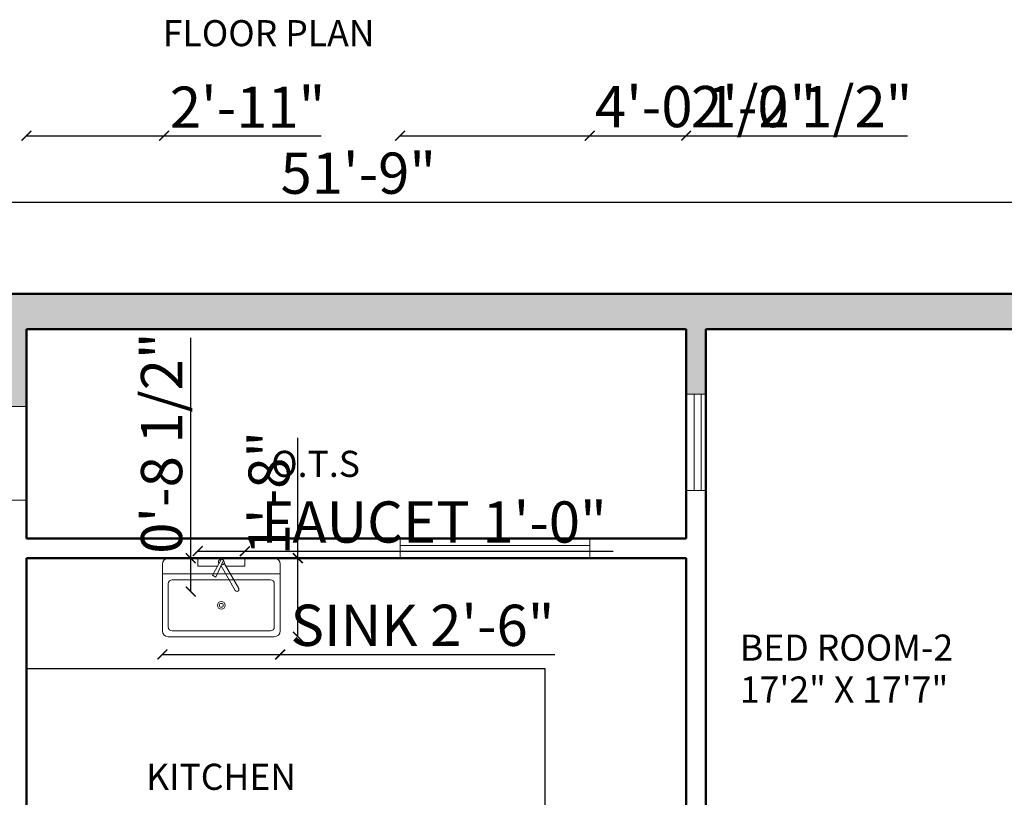
# Model space of a CAD drawing. Units: inches. Extents: x 1549 to 2410, y 1378 to 2139.
# Tile 5 of 6: x 1913 to 2164, y 1941 to 2139. Entities that reach past the tile are written whole.
import ezdxf

# ---------------------------------------------------------------- set-up
doc = ezdxf.new("R2010")
doc.units = ezdxf.units.IN
for name, color, linetype, lineweight in [('A-ANNO-DIMS', 2, 'Continuous', 18), ('A-ANNO-TEXT', 7, 'Continuous', 25), ('A-AREA-IDEN', 7, 'Continuous', 18), ('A-FLOR-CASE', 30, 'Continuous', 25), ('A-FLOR-FIXT', 9, 'Continuous', 18), ('A-WALL', 7, 'Continuous', 50), ('WINDOW', 2, 'Continuous', 18)]:
    doc.layers.add(name, color=color, linetype=linetype, lineweight=lineweight)
doc.layers.add('A-WALL-PATT', color=18, linetype='Continuous', lineweight=13, true_color=0x000000)
doc.styles.get("Standard").update_dxf_attribs({"font": 'arial.ttf'})
doc.dimstyles.new('ISO-25', dxfattribs={"dimtxt": 10.5, "dimasz": 2.5, "dimexe": 1.25, "dimexo": 0.625, "dimtad": 1, "dimdec": 0, "dimlunit": 4, "dimtxsty": 'Standard', "dimblk": 'ARCHTICK', "dimcen": 2.5, "dimse1": 1, "dimse2": 1, "dimclrd": 1, "dimclrt": 3, "dimadec": 0, "dimazin": 0, "dimtfac": 1, "dimtdec": 0, "dimtmove": 0, "dimatfit": 3, "dimfxl": 1, "dimarcsym": 0})

# ---------------------------------------------------------------- blocks, each defined once
blk = doc.blocks.new('Sink-single - 30 in top')
blk.add_line((-15, -3.999996), (15, -3.999996))
for points in [[(-13.5, 0), (13.5, 0)], [(-15, -18.499996), (-15, -1.5)], [(15, -1.5), (15, -18.499996)], [(-13.5, -17.499996), (-13.5, -6.499996)], [(-12.5, -5.499996), (12.5, -5.499996)], [(13.5, -6.499996), (13.5, -17.499996)], [(13.5, -19.999996), (-13.5, -19.999996)], [(12.5, -18.499996), (-12.5, -18.499996)]]:
    blk.add_lwpolyline(points)
for radius in [1, 0.5]:
    blk.add_circle((0, -11.999996), radius)
for centre, radius, start, end in [((-13.5, -1.5), 1.5, 90, 180), ((13.5, -1.5), 1.5, 0, 90), ((-12.5, -6.499996), 1, 90, 180), ((12.5, -6.499996), 1, 0, 90), ((-12.5, -17.499996), 1, 180, 270), ((12.5, -17.499996), 1, 270, 0), ((-13.5, -18.499996), 1.5, 180, 270), ((13.5, -18.499996), 1.5, 270, 0)]:
    blk.add_arc(centre, radius, start, end)
blk = doc.blocks.new('Faucet - single handle top')
for p, q in [((0.08, -0.26), (-2.26, -4.34)), ((-1.37, -4.79), (0.55, -0.5)), ((-0.06, -1.9), (3.57, -8.18)), ((4.43, -7.68), (0.72, -1.24)), ((-2.26, -4.34), (-1.37, -4.79))]:
    blk.add_line(p, q)
for points in [[(-0.92, -2), (-6, -2), (-6, 0), (6, 0), (6, -2), (1.16, -2)], [(-0.01, -2), (-0.12, -2)]]:
    blk.add_lwpolyline(points)
for centre, radius, start, end in [((0, -1), 0.75, 269.2246, 216.2304), ((4, -7.93), 0.5, 210, 30)]:
    blk.add_arc(centre, radius, start, end)
blk = doc.blocks.new('_ArchTick')
at = {"color": 0, "linetype": 'ByBlock', "const_width": 0.15}
blk.add_lwpolyline([(-0.5, -0.5), (0.5, 0.5)], dxfattribs=at)
blk = doc.blocks.new('*D13')
at = {"layer": 'A-ANNO-DIMS', "color": 0, "lineweight": -2, "transparency": 16777216}
blk.add_line((1688.62, 2092.38), (2309.62, 2092.38), dxfattribs=at)
at = {"layer": 'Defpoints', "color": 0, "transparency": 16777216}
for p in [(2309.62, 2092.38), (1688.62, 2069.01), (2309.62, 2069.01)]:
    blk.add_point(p, dxfattribs=at)
at = {"layer": 'A-ANNO-DIMS', "color": 0, "lineweight": -2, "transparency": 16777216, "xscale": 2.5, "yscale": 2.5, "zscale": 2.5, "rotation": 180}
blk.add_blockref('_ArchTick', (1688.62, 2092.38), dxfattribs=at)
at = {"layer": 'A-ANNO-DIMS', "color": 0, "lineweight": -2, "transparency": 16777216, "xscale": 2.5, "yscale": 2.5, "zscale": 2.5}
blk.add_blockref('_ArchTick', (2309.62, 2092.38), dxfattribs=at)
at = {"layer": 'A-ANNO-DIMS', "color": 0, "transparency": 16777216, "insert": (1999.12, 2098.36), "char_height": 10.5, "attachment_point": 5}
blk.add_mtext('51\'-9"', dxfattribs=at)
blk = doc.blocks.new('*D19')
at = {"layer": 'A-ANNO-DIMS', "color": 1, "lineweight": -2, "transparency": 16777216}
for p, q in [((1949.24, 1977.16), (1979.24, 1977.16)), ((1979.24, 1977.16), (2049.17, 1977.16))]:
    blk.add_line(p, q, dxfattribs=at)
at = {"layer": 'Defpoints', "color": 0, "transparency": 16777216}
for p in [(1949.24, 1981.66), (1979.24, 1981.66), (1979.24, 1977.16)]:
    blk.add_point(p, dxfattribs=at)
at = {"layer": 'A-ANNO-DIMS', "color": 1, "lineweight": -2, "transparency": 16777216, "xscale": 2.5, "yscale": 2.5, "zscale": 2.5, "rotation": 180}
blk.add_blockref('_ArchTick', (1949.24, 1977.16), dxfattribs=at)
at = {"layer": 'A-ANNO-DIMS', "color": 1, "lineweight": -2, "transparency": 16777216, "xscale": 2.5, "yscale": 2.5, "zscale": 2.5}
blk.add_blockref('_ArchTick', (1979.24, 1977.16), dxfattribs=at)
at = {"layer": 'A-ANNO-DIMS', "color": 3, "transparency": 16777216, "insert": (2015.46, 1983.22), "char_height": 10.5, "attachment_point": 5}
blk.add_mtext('SINK 2\'-6"', dxfattribs=at)
blk = doc.blocks.new('*D20')
at = {"layer": 'A-ANNO-DIMS', "color": 1, "lineweight": -2, "transparency": 16777216}
for p, q in [((1983.74, 2001.66), (1983.74, 2032.34)), ((1983.74, 1981.66), (1983.74, 2001.66))]:
    blk.add_line(p, q, dxfattribs=at)
at = {"layer": 'Defpoints', "color": 0, "transparency": 16777216}
for p in [(1979.24, 2001.66), (1983.74, 2001.66), (1979.24, 1981.66)]:
    blk.add_point(p, dxfattribs=at)
at = {"layer": 'A-ANNO-DIMS', "color": 1, "lineweight": -2, "transparency": 16777216, "xscale": 2.5, "yscale": 2.5, "zscale": 2.5}
for p, rotation in [((1983.74, 2001.66), 90), ((1983.74, 1981.66), 270)]:
    blk.add_blockref('_ArchTick', p, dxfattribs=dict(at, rotation=rotation))
at = {"layer": 'A-ANNO-DIMS', "color": 3, "transparency": 16777216, "insert": (1977.76, 2018.25), "char_height": 10.5, "attachment_point": 5, "rotation": 90}
blk.add_mtext('1\'-8"', dxfattribs=at)
blk = doc.blocks.new('*D21')
at = {"layer": 'A-ANNO-DIMS', "color": 1, "lineweight": -2, "transparency": 16777216}
for p, q in [((1958.24, 2003.46), (1970.24, 2003.46)), ((1970.24, 2003.46), (2064.06, 2003.46))]:
    blk.add_line(p, q, dxfattribs=at)
at = {"layer": 'Defpoints', "color": 0, "transparency": 16777216}
for p in [(1970.24, 2003.46), (1958.24, 2001.66), (1970.24, 2001.66)]:
    blk.add_point(p, dxfattribs=at)
at = {"layer": 'A-ANNO-DIMS', "color": 1, "lineweight": -2, "transparency": 16777216, "xscale": 2.5, "yscale": 2.5, "zscale": 2.5, "rotation": 180}
blk.add_blockref('_ArchTick', (1958.24, 2003.46), dxfattribs=at)
at = {"layer": 'A-ANNO-DIMS', "color": 1, "lineweight": -2, "transparency": 16777216, "xscale": 2.5, "yscale": 2.5, "zscale": 2.5}
blk.add_blockref('_ArchTick', (1970.24, 2003.46), dxfattribs=at)
at = {"layer": 'A-ANNO-DIMS', "color": 3, "transparency": 16777216, "insert": (2018.4, 2009.52), "char_height": 10.5, "attachment_point": 5}
blk.add_mtext('FAUCET 1\'-0"', dxfattribs=at)
blk = doc.blocks.new('*D22')
at = {"layer": 'A-ANNO-DIMS', "color": 1, "lineweight": -2, "transparency": 16777216}
for p, q in [((1956.44, 2001.66), (1956.44, 2057.79)), ((1956.44, 1993.17), (1956.44, 2001.66))]:
    blk.add_line(p, q, dxfattribs=at)
at = {"layer": 'Defpoints', "color": 0, "transparency": 16777216}
for p in [(1956.44, 2001.66), (1958.24, 2001.66), (1958.24, 1993.17)]:
    blk.add_point(p, dxfattribs=at)
at = {"layer": 'A-ANNO-DIMS', "color": 1, "lineweight": -2, "transparency": 16777216, "xscale": 2.5, "yscale": 2.5, "zscale": 2.5}
for p, rotation in [((1956.44, 2001.66), 90), ((1956.44, 1993.17), 270)]:
    blk.add_blockref('_ArchTick', p, dxfattribs=dict(at, rotation=rotation))
at = {"layer": 'A-ANNO-DIMS', "color": 3, "transparency": 16777216, "insert": (1950.39, 2030.98), "char_height": 10.5, "attachment_point": 5, "rotation": 90}
blk.add_mtext('0\'-8 1/2"', dxfattribs=at)
blk = doc.blocks.new('*D48')
at = {"layer": 'A-ANNO-DIMS', "color": 1, "lineweight": -2, "transparency": 16777216}
for p, q in [((2400.7, 2060.01), (2400.7, 2006.66)), ((2400.7, 2006.66), (2400.7, 1950.11))]:
    blk.add_line(p, q, dxfattribs=at)
at = {"layer": 'Defpoints', "color": 0, "transparency": 16777216}
for p in [(1914.62, 2060.01), (1914.62, 2006.66), (2400.7, 2006.66)]:
    blk.add_point(p, dxfattribs=at)
at = {"layer": 'A-ANNO-DIMS', "color": 1, "lineweight": -2, "transparency": 16777216, "xscale": 2.5, "yscale": 2.5, "zscale": 2.5}
for p, rotation in [((2400.7, 2060.01), 90), ((2400.7, 2006.66), 270)]:
    blk.add_blockref('_ArchTick', p, dxfattribs=dict(at, rotation=rotation))
at = {"layer": 'A-ANNO-DIMS', "color": 3, "transparency": 16777216, "insert": (2394.65, 1977.14), "char_height": 10.5, "attachment_point": 5, "rotation": 90}
blk.add_mtext('4\'-5 1/2"', dxfattribs=at)
blk = doc.blocks.new('*D51')
at = {"layer": 'A-ANNO-DIMS', "color": 1, "lineweight": -2, "transparency": 16777216}
for p, q in [((1648.37, 2001.66), (1648.37, 2033.51)), ((1648.37, 1973.56), (1648.37, 2001.66))]:
    blk.add_line(p, q, dxfattribs=at)
at = {"layer": 'Defpoints', "color": 0, "transparency": 16777216}
for p in [(1648.37, 2001.66), (1914.62, 2001.66), (1914.62, 1973.56)]:
    blk.add_point(p, dxfattribs=at)
at = {"layer": 'A-ANNO-DIMS', "color": 1, "lineweight": -2, "transparency": 16777216, "xscale": 2.5, "yscale": 2.5, "zscale": 2.5}
for p, rotation in [((1648.37, 2001.66), 90), ((1648.37, 1973.56), 270)]:
    blk.add_blockref('_ArchTick', p, dxfattribs=dict(at, rotation=rotation))
at = {"layer": 'A-ANNO-DIMS', "color": 3, "transparency": 16777216, "insert": (1642.47, 2018.83), "char_height": 10.5, "attachment_point": 5, "rotation": 90}
blk.add_mtext('2\'-4"', dxfattribs=at)
blk = doc.blocks.new('*D53')
at = {"layer": 'A-ANNO-DIMS', "color": 1, "lineweight": -2, "transparency": 16777216}
for p, q in [((2009.78, 2109.26), (2058.05, 2109.26)), ((2058.05, 2109.26), (2114.6, 2109.26))]:
    blk.add_line(p, q, dxfattribs=at)
at = {"layer": 'Defpoints', "color": 0, "transparency": 16777216}
for p in [(2058.05, 2109.26), (2009.78, 2006.66), (2058.05, 2006.66)]:
    blk.add_point(p, dxfattribs=at)
at = {"layer": 'A-ANNO-DIMS', "color": 1, "lineweight": -2, "transparency": 16777216, "xscale": 2.5, "yscale": 2.5, "zscale": 2.5, "rotation": 180}
blk.add_blockref('_ArchTick', (2009.78, 2109.26), dxfattribs=at)
at = {"layer": 'A-ANNO-DIMS', "color": 1, "lineweight": -2, "transparency": 16777216, "xscale": 2.5, "yscale": 2.5, "zscale": 2.5}
blk.add_blockref('_ArchTick', (2058.05, 2109.26), dxfattribs=at)
at = {"layer": 'A-ANNO-DIMS', "color": 3, "transparency": 16777216, "insert": (2087.57, 2115.32), "char_height": 10.5, "attachment_point": 5}
blk.add_mtext('4\'-0 1/2"', dxfattribs=at)
blk = doc.blocks.new('*D57')
at = {"layer": 'A-ANNO-DIMS', "color": 1, "lineweight": -2, "transparency": 16777216}
for p, q in [((1914.62, 2109.26), (1949.68, 2109.26)), ((1949.68, 2109.26), (1989.68, 2109.26))]:
    blk.add_line(p, q, dxfattribs=at)
at = {"layer": 'Defpoints', "color": 0, "transparency": 16777216}
for p in [(1949.68, 2109.26), (1914.62, 2001.66), (1949.68, 2001.23)]:
    blk.add_point(p, dxfattribs=at)
at = {"layer": 'A-ANNO-DIMS', "color": 1, "lineweight": -2, "transparency": 16777216, "xscale": 2.5, "yscale": 2.5, "zscale": 2.5, "rotation": 180}
blk.add_blockref('_ArchTick', (1914.62, 2109.26), dxfattribs=at)
at = {"layer": 'A-ANNO-DIMS', "color": 1, "lineweight": -2, "transparency": 16777216, "xscale": 2.5, "yscale": 2.5, "zscale": 2.5}
blk.add_blockref('_ArchTick', (1949.68, 2109.26), dxfattribs=at)
at = {"layer": 'A-ANNO-DIMS', "color": 3, "transparency": 16777216, "insert": (1970.93, 2115.16), "char_height": 10.5, "attachment_point": 5}
blk.add_mtext('2\'-11"', dxfattribs=at)
blk = doc.blocks.new('*D58')
at = {"layer": 'A-ANNO-DIMS', "color": 1, "lineweight": -2, "transparency": 16777216}
for p, q in [((2058.05, 2109.26), (2082.62, 2109.26)), ((2082.62, 2109.26), (2138.93, 2109.26))]:
    blk.add_line(p, q, dxfattribs=at)
at = {"layer": 'Defpoints', "color": 0, "transparency": 16777216}
for p in [(2082.62, 2109.26), (2058.05, 2006.66), (2082.62, 2006.66)]:
    blk.add_point(p, dxfattribs=at)
at = {"layer": 'A-ANNO-DIMS', "color": 1, "lineweight": -2, "transparency": 16777216, "xscale": 2.5, "yscale": 2.5, "zscale": 2.5, "rotation": 180}
blk.add_blockref('_ArchTick', (2058.05, 2109.26), dxfattribs=at)
at = {"layer": 'A-ANNO-DIMS', "color": 1, "lineweight": -2, "transparency": 16777216, "xscale": 2.5, "yscale": 2.5, "zscale": 2.5}
blk.add_blockref('_ArchTick', (2082.62, 2109.26), dxfattribs=at)
at = {"layer": 'A-ANNO-DIMS', "color": 3, "transparency": 16777216, "insert": (2112.02, 2115.32), "char_height": 10.5, "attachment_point": 5}
blk.add_mtext('2\'-0 1/2"', dxfattribs=at)
blk = doc.blocks.new('*D66')
at = {"layer": 'A-ANNO-DIMS', "color": 1, "lineweight": -2, "transparency": 16777216}
for p, q in [((2400.7, 2043.41), (2400.7, 2099.71)), ((2400.7, 2018.94), (2400.7, 2043.41))]:
    blk.add_line(p, q, dxfattribs=at)
at = {"layer": 'Defpoints', "color": 0, "transparency": 16777216}
for p in [(2087.62, 2043.41), (2400.7, 2043.41), (2087.62, 2018.94)]:
    blk.add_point(p, dxfattribs=at)
at = {"layer": 'A-ANNO-DIMS', "color": 1, "lineweight": -2, "transparency": 16777216, "xscale": 2.5, "yscale": 2.5, "zscale": 2.5}
for p, rotation in [((2400.7, 2043.41), 90), ((2400.7, 2018.94), 270)]:
    blk.add_blockref('_ArchTick', p, dxfattribs=dict(at, rotation=rotation))
at = {"layer": 'A-ANNO-DIMS', "color": 3, "transparency": 16777216, "insert": (2394.65, 2072.81), "char_height": 10.5, "attachment_point": 5, "rotation": 90}
blk.add_mtext('2\'-0 1/2"', dxfattribs=at)

msp = doc.modelspace()

# ---------------------------------------------------------------- hatches: boundary and pattern name
at = {"layer": 'A-WALL-PATT'}
h = msp.add_hatch(color=256, dxfattribs=at)
h.dxf.hatch_style = 1
h.paths.add_polyline_path([(1760, 2069.01), (1688.62, 2069.01), (1688.62, 2003.68), (1697.62, 2003.68), (1697.62, 2060.01), (1760, 2060.01)])
h.paths.add_polyline_path([(2309.62, 2069.01), (1807.68, 2069.01), (1807.68, 2060.01), (1909.62, 2060.01), (1909.62, 2040.27), (1914.62, 2040.27), (1914.62, 2060.01), (2082.62, 2060.01), (2082.62, 2043.41), (2087.62, 2043.41), (2087.62, 2060.01), (2300.62, 2060.01), (2300.62, 2006.22), (2309.62, 2006.22)])
h.paths.add_polyline_path([(1914.62, 1607.36), (1909.62, 1607.36), (1909.62, 1437.01), (1914.62, 1437.01)])
h.paths.add_polyline_path([(1697.62, 1536.06), (1688.62, 1536.06), (1688.62, 1428.01), (1745.28, 1428.01), (1745.28, 1437.01), (1697.62, 1437.01)])
h.paths.add_polyline_path([(2130.61, 1437.01), (2082.62, 1437.01), (2082.62, 1428.01), (2130.61, 1428.01)])
h.paths.add_polyline_path([(2309.62, 1544.51), (2302.25, 1544.51), (2302.25, 1524.81), (2300.62, 1524.81), (2300.62, 1523.51), (2302.17, 1523.51), (2302.17, 1503.88), (2300.62, 1503.88), (2300.62, 1437.01), (2193.34, 1437.01), (2193.34, 1428.01), (2309.62, 1428.01)])
h.paths.add_polyline_path([(2309.62, 1708.66), (2300.62, 1708.66), (2300.62, 1657.01), (2293.7, 1657.01), (2293.7, 1652.01), (2300.62, 1652.01), (2300.62, 1611.18), (2302.17, 1611.18), (2302.17, 1597.64), (2309.62, 1597.64)])
h.paths.add_polyline_path([(2309.62, 1777.38), (2300.62, 1777.38), (2300.62, 1737.9), (2309.62, 1737.9)])
h.paths.add_polyline_path([(2300.62, 1757.01), (2168.62, 1757.01), (2168.62, 1795.96), (2163.62, 1795.96), (2163.62, 1657.01), (2082.62, 1657.01), (2082.62, 1641.99), (2087.62, 1641.99), (2087.62, 1652.01), (2253.7, 1652.01), (2253.7, 1657.01), (2168.62, 1657.01), (2168.62, 1752.01), (2300.62, 1752.01)])
h.paths.add_polyline_path([(2309.62, 1957.79), (2300.62, 1957.79), (2300.62, 1935.33), (2300.62, 1824.93), (2309.62, 1824.93)])
h.paths.add_polyline_path([(2300.62, 1849.01), (2137.17, 1849.01), (2137.17, 1844.01), (2163.62, 1844.01), (2163.62, 1835.96), (2168.62, 1835.96), (2168.62, 1844.01), (2300.62, 1844.01)])
h.paths.add_polyline_path([(2211.06, 1800.23), (2261.76, 1800.23), (2261.76, 1810.41), (2211.06, 1810.41)], flags=9)
h.paths.add_polyline_path([(2211.1, 1811.05), (2239.18, 1811.05), (2239.18, 1821.02), (2211.1, 1821.02)], flags=9)
h.paths.add_polyline_path([(2187.84, 1718.73), (2233.38, 1718.73), (2233.38, 1728.91), (2187.84, 1728.91)], flags=25)
h.paths.add_polyline_path([(2187.88, 1729.56), (2215.96, 1729.56), (2215.96, 1739.52), (2187.88, 1739.52)], flags=25)
h.paths.add_polyline_path([(1720.01, 1609.74), (1775.87, 1609.74), (1775.87, 1619.93), (1720.01, 1619.93)], flags=9)
h.paths.add_polyline_path([(1719.99, 1620.4), (1782.23, 1620.4), (1782.23, 1630.72), (1719.99, 1630.72)], flags=9)
h.paths.add_polyline_path([(2092.97, 1541.04), (2148.83, 1541.04), (2148.83, 1551.23), (2092.97, 1551.23)], flags=9)
h.paths.add_polyline_path([(2092.94, 1551.69), (2155.19, 1551.69), (2155.19, 1562.02), (2092.94, 1562.02)], flags=9)
h.paths.add_polyline_path([(1759.73, 1747.67), (1815.59, 1747.67), (1815.59, 1757.85), (1759.73, 1757.85)], flags=9)
h.paths.add_polyline_path([(1759.71, 1758.32), (1790.48, 1758.32), (1790.48, 1768.63), (1759.71, 1768.63)], flags=9)
h.paths.add_polyline_path([(1940.79, 1793.43), (1996.65, 1793.43), (1996.65, 1803.61), (1940.79, 1803.61)], flags=9)
h.paths.add_polyline_path([(1940.77, 1804.08), (2006.11, 1804.08), (2006.11, 1814.4), (1940.77, 1814.4)], flags=9)
h.paths.add_polyline_path([(2094.62, 1963.23), (2150.43, 1963.23), (2150.43, 1973.25), (2094.62, 1973.25)], flags=9)
h.paths.add_polyline_path([(2094.57, 1973.75), (2156.81, 1973.75), (2156.81, 1984.07), (2094.57, 1984.07)], flags=9)
h.paths.add_polyline_path([(1943.36, 1930.19), (2000.28, 1930.19), (2000.28, 1940.37), (1943.36, 1940.37)], flags=9)
h.paths.add_polyline_path([(1943.34, 1940.85), (1987.53, 1940.85), (1987.53, 1951.15), (1943.34, 1951.15)], flags=9)
h.paths.add_polyline_path([(1803.94, 1971.5), (1857.22, 1971.5), (1857.22, 1981.68), (1803.94, 1981.68)], flags=9)
h.paths.add_polyline_path([(1803.92, 1982.16), (1866.16, 1982.16), (1866.16, 1992.47), (1803.92, 1992.47)], flags=9)

# ---------------------------------------------------------------- linework, layer by layer
at = {"layer": 'A-FLOR-CASE'}
for p, q in [((1914.62, 1973.56), (2046.65, 1973.56)), ((2046.65, 1973.56), (2046.65, 1849.01))]:
    msp.add_line(p, q, dxfattribs=at)
at = {"layer": 'A-WALL'}
for p, q in [((1914.62, 2006.66), (1914.62, 2060.01)), ((1914.62, 2060.01), (2082.62, 2060.01)), ((2082.62, 2006.66), (2082.62, 2060.01)), ((2087.62, 1849.01), (2087.62, 2060.01)), ((2087.62, 2060.01), (2300.62, 2060.01)), ((1914.62, 2006.66), (2082.62, 2006.66)), ((1914.62, 2001.66), (2082.62, 2001.66)), ((1914.62, 1849.01), (1914.62, 2001.66)), ((2082.62, 1849.01), (2082.62, 2001.66))]:
    msp.add_line(p, q, dxfattribs=at)
msp.add_lwpolyline([(1914.62, 1428.01), (1688.62, 1428.01), (1688.62, 2069.01), (2309.62, 2069.01), (2309.62, 1428.01), (2082.62, 1428.01)], dxfattribs=at)
at = {"layer": 'WINDOW'}
for p, q in [((2087.62, 2043.41), (2082.62, 2043.41)), ((2082.62, 2043.41), (2082.62, 2018.94)), ((2084.66, 2018.94), (2084.66, 2043.41)), ((2086.45, 2018.94), (2086.45, 2043.41)), ((2087.62, 2018.94), (2087.62, 2043.41)), ((1914.62, 2040.27), (1909.62, 2040.27)), ((1914.62, 2016.45), (1914.62, 2040.27)), ((2082.62, 2018.94), (2087.62, 2018.94)), ((1909.62, 2016.45), (1914.62, 2016.45)), ((2009.78, 2006.66), (2009.78, 2001.66)), ((2058.05, 2006.66), (2009.78, 2006.66)), ((2058.05, 2001.66), (2058.05, 2006.66)), ((2058.05, 2004.93), (2009.78, 2004.93)), ((2058.05, 2003.43), (2009.78, 2003.43)), ((2009.78, 2001.66), (2058.05, 2001.66))]:
    msp.add_line(p, q, dxfattribs=at)

# ---------------------------------------------------------------- block references
at = {"layer": 'A-FLOR-FIXT'}
for name in ['Sink-single - 30 in top', 'Faucet - single handle top']:
    msp.add_blockref(name, (1964.24, 2001.66), dxfattribs=at)

# ---------------------------------------------------------------- texts
at = {"layer": 'A-ANNO-TEXT'}
msp.add_text('FLOOR PLAN', height=6.645, dxfattribs=at).set_placement((1949.36, 2132.05))
at = {"layer": 'A-AREA-IDEN'}
for s, height, p in [('O.T.S', 6.645, (1976.95, 2022.37)), ('BED ROOM-2', 6.645, (2096.29, 1975.58)), ('17\'2" X 17\'7"', 6.6455, (2096.29, 1964.91)), ('KITCHEN', 6.645, (1945.06, 1942.68))]:
    msp.add_text(s, height=height, dxfattribs=at).set_placement(p)

# ---------------------------------------------------------------- dimensions: what is measured, and where the dimension line sits
at = {"layer": 'A-ANNO-DIMS'}
for base, p1, p2, override, picture, middle in [((2058.05, 2109.26), (2009.78, 2006.66), (2058.05, 2006.66), {"dimdec": 1, "dimlfac": 1, "dimrnd": 0, "dimzin": 1, "dimdsep": 46, "dimlunit": 4, "dimfrac": 2}, '*D53', (2087.57, 2115.32)), ((2082.62, 2109.26), (2058.05, 2006.66), (2082.62, 2006.66), {"dimdec": 1, "dimlfac": 1, "dimrnd": 0, "dimzin": 1, "dimdsep": 46, "dimlunit": 4, "dimfrac": 2}, '*D58', (2112.02, 2115.32)), ((1949.68, 2109.26), (1914.62, 2001.66), (1949.68, 2001.23), {"dimdec": 1, "dimlfac": 1, "dimrnd": 0, "dimzin": 1, "dimdsep": 46, "dimlunit": 4, "dimfrac": 2}, '*D57', (1970.93, 2115.16)), ((2309.62, 2092.38), (1688.62, 2069.01), (2309.62, 2069.01), {"dimclrd": 0, "dimclre": 0, "dimclrt": 0}, '*D13', (1999.12, 2098.36))]:
    dim = msp.add_linear_dim(base=base, p1=p1, p2=p2, dimstyle='ISO-25', override=override, dxfattribs=at)
    dim.commit()
    dim.dimension.update_dxf_attribs({"geometry": picture, "text_midpoint": middle})
for base, p1, p2, picture, middle in [((2400.7, 2043.41), (2087.62, 2018.94), (2087.62, 2043.41), '*D66', (2394.65, 2072.81)), ((2400.7045, 2006.6646), (1914.6182, 2060.0143), (1914.6182, 2006.6646), '*D48', (2394.6504, 1977.1391)), ((1956.44, 2001.66), (1958.24, 1993.17), (1958.24, 2001.66), '*D22', (1950.39, 2030.98)), ((1648.37, 2001.66), (1914.62, 1973.56), (1914.62, 2001.66), '*D51', (1642.47, 2018.83)), ((1983.74, 2001.66), (1979.24, 1981.66), (1979.24, 2001.66), '*D20', (1977.76, 2018.25))]:
    dim = msp.add_linear_dim(base=base, p1=p1, p2=p2, angle=90, dimstyle='ISO-25', override={"dimdec": 1, "dimlfac": 1, "dimrnd": 0, "dimzin": 1, "dimdsep": 46, "dimlunit": 4, "dimfrac": 2}, dxfattribs=at)
    dim.commit()
    dim.dimension.update_dxf_attribs({"geometry": picture, "text_midpoint": middle})
for base, p1, p2, text, picture, middle in [((1970.24, 2003.46), (1958.24, 2001.66), (1970.24, 2001.66), 'FAUCET <>', '*D21', (2018.4, 2009.52)), ((1979.24, 1977.16), (1949.24, 1981.66), (1979.24, 1981.66), 'SINK <>', '*D19', (2015.46, 1983.22))]:
    dim = msp.add_linear_dim(base=base, p1=p1, p2=p2, text=text, dimstyle='ISO-25', override={"dimdec": 1, "dimlfac": 1, "dimrnd": 0, "dimzin": 1, "dimdsep": 46, "dimlunit": 4, "dimfrac": 2}, dxfattribs=at)
    dim.commit()
    dim.dimension.update_dxf_attribs({"geometry": picture, "text_midpoint": middle})

doc.saveas('drawing.dxf')
